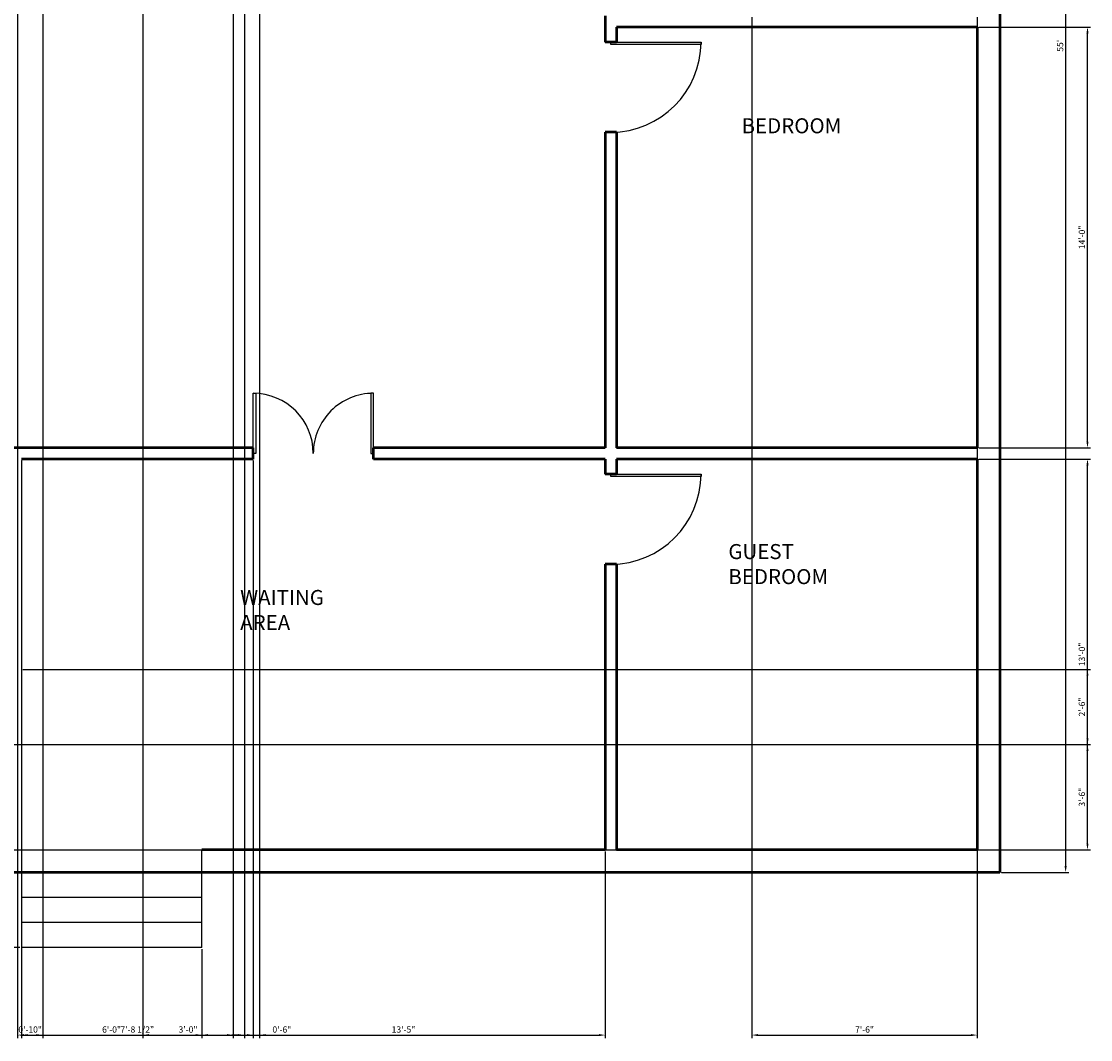
# Model space of a CAD drawing. Units: inches. Extents: x 877 to 2164, y 771 to 1603.
# Tile 3 of 6: x 1281 to 1708, y 771 to 1177. Entities that reach past the tile are written whole.
import ezdxf

# ---------------------------------------------------------------- set-up
doc = ezdxf.new("R2010")
doc.units = ezdxf.units.IN
for name, color, linetype, lineweight in [('A-ANNO-DIMS', 2, 'Continuous', 18), ('A-AREA-IDEN', 7, 'Continuous', 25), ('A-DOOR', 5, 'Continuous', 25), ('A-FLOR-STRS', 7, 'Continuous', 25), ('A-WALL', 7, 'Continuous', 50)]:
    doc.layers.add(name, color=color, linetype=linetype, lineweight=lineweight)
doc.styles.get("Standard").update_dxf_attribs({"font": 'arial.ttf'})
doc.dimstyles.new('ISO-25', dxfattribs={"dimtxt": 2.5, "dimasz": 2.5, "dimexe": 1.25, "dimexo": 0.625, "dimtad": 1, "dimdec": 0, "dimlunit": 4, "dimtxsty": 'Standard', "dimcen": 2.5, "dimadec": 0, "dimazin": 0, "dimtfac": 1, "dimtdec": 0, "dimtmove": 0, "dimatfit": 3, "dimfxl": 1, "dimarcsym": 0})

# ---------------------------------------------------------------- blocks, each defined once
blk = doc.blocks.new('*D2')
at = {"layer": 'A-ANNO-DIMS', "color": 0, "lineweight": -2, "transparency": 16777216}
for p, q in [((1672.52, 1497.62), (1699.4, 1497.62)), ((1698.15, 1495.12), (1698.15, 840.12)), ((1672.52, 837.62), (1699.4, 837.62))]:
    blk.add_line(p, q, dxfattribs=at)
at = {"layer": 'A-ANNO-DIMS', "color": 0, "transparency": 16777216}
for points in [[(1697.73, 1495.12), (1698.57, 1495.12), (1698.15, 1497.62)], [(1697.73, 840.12), (1698.57, 840.12), (1698.15, 837.62)]]:
    blk.add_solid(points, dxfattribs=at)
at = {"layer": 'Defpoints', "color": 0, "transparency": 16777216}
for p in [(1671.89, 1497.62), (1671.89, 837.62), (1698.15, 837.62)]:
    blk.add_point(p, dxfattribs=at)
at = {"layer": 'A-ANNO-DIMS', "color": 0, "transparency": 16777216, "insert": (1696.26, 1167.62), "char_height": 2.5, "attachment_point": 5, "rotation": 90}
blk.add_mtext("55'", dxfattribs=at)
blk = doc.blocks.new('DOOR-SINGLE-36IN')
blk.add_lwpolyline([(0, 0), (0, 1), (36, 1), (36, 0)], close=True)
blk.add_arc((36, 0), 36, 90, 180)
blk = doc.blocks.new('DOOR-DOUBLE-48IN')
for points in [[(0, 0), (1, 0), (1, 24), (0, 24)], [(48, 0), (47, 0), (47, 24), (48, 24)]]:
    blk.add_lwpolyline(points, close=True)
for centre, start, end in [((0, 24), 270, 0), ((48, 24), 180, 270)]:
    blk.add_arc(centre, 24, start, end)
blk = doc.blocks.new('*D18')
at = {"layer": 'A-ANNO-DIMS', "color": 0, "lineweight": -2, "transparency": 16777216}
for p, q in [((1572.89, 1179), (1572.89, 771.4)), ((1662.89, 1179), (1662.89, 771.4)), ((1575.39, 772.65), (1660.39, 772.65))]:
    blk.add_line(p, q, dxfattribs=at)
at = {"layer": 'A-ANNO-DIMS', "color": 0, "transparency": 16777216}
for points in [[(1575.39, 773.06), (1575.39, 772.23), (1572.89, 772.65)], [(1660.39, 773.06), (1660.39, 772.23), (1662.89, 772.65)]]:
    blk.add_solid(points, dxfattribs=at)
at = {"layer": 'Defpoints', "color": 0, "transparency": 16777216}
for p in [(1572.89, 1179.62), (1662.89, 1179.62), (1662.89, 772.65)]:
    blk.add_point(p, dxfattribs=at)
at = {"layer": 'A-ANNO-DIMS', "color": 0, "transparency": 16777216, "insert": (1617.89, 774.55), "char_height": 2.5, "attachment_point": 5}
blk.add_mtext('7\'-6"', dxfattribs=at)
blk = doc.blocks.new('*D22')
at = {"layer": 'A-ANNO-DIMS', "color": 0, "lineweight": -2, "transparency": 16777216}
for p, q in [((1663.52, 1175.12), (1708.12, 1175.12)), ((1706.87, 1009.62), (1706.87, 1172.62)), ((1663.52, 1007.12), (1708.12, 1007.12))]:
    blk.add_line(p, q, dxfattribs=at)
at = {"layer": 'A-ANNO-DIMS', "color": 0, "transparency": 16777216}
for points in [[(1706.45, 1172.62), (1707.29, 1172.62), (1706.87, 1175.12)], [(1706.45, 1009.62), (1707.29, 1009.62), (1706.87, 1007.12)]]:
    blk.add_solid(points, dxfattribs=at)
at = {"layer": 'Defpoints', "color": 0, "transparency": 16777216}
for p in [(1662.89, 1175.12), (1706.87, 1175.12), (1662.89, 1007.12)]:
    blk.add_point(p, dxfattribs=at)
at = {"layer": 'A-ANNO-DIMS', "color": 0, "transparency": 16777216, "insert": (1704.97, 1091.12), "char_height": 2.5, "attachment_point": 5, "rotation": 90}
blk.add_mtext('14\'-0"', dxfattribs=at)
blk = doc.blocks.new('*D23')
at = {"layer": 'A-ANNO-DIMS', "color": 0, "lineweight": -2, "transparency": 16777216}
for p, q in [((1663.52, 1002.62), (1708.12, 1002.62)), ((1706.87, 849.12), (1706.87, 1000.12)), ((1663.52, 846.62), (1708.12, 846.62))]:
    blk.add_line(p, q, dxfattribs=at)
at = {"layer": 'A-ANNO-DIMS', "color": 0, "transparency": 16777216}
for points in [[(1706.45, 1000.12), (1707.29, 1000.12), (1706.87, 1002.62)], [(1706.45, 849.12), (1707.29, 849.12), (1706.87, 846.62)]]:
    blk.add_solid(points, dxfattribs=at)
at = {"layer": 'Defpoints', "color": 0, "transparency": 16777216}
for p in [(1662.89, 1002.62), (1706.87, 1002.62), (1662.89, 846.62)]:
    blk.add_point(p, dxfattribs=at)
at = {"layer": 'A-ANNO-DIMS', "color": 0, "transparency": 16777216, "insert": (1704.97, 924.62), "char_height": 2.5, "attachment_point": 5, "rotation": 90}
blk.add_mtext('13\'-0"', dxfattribs=at)
blk = doc.blocks.new('*D27')
at = {"layer": 'A-ANNO-DIMS', "color": 0, "lineweight": -2, "transparency": 16777216}
for p, q in [((1514.39, 846), (1514.39, 771.4)), ((1353.39, 807), (1353.39, 771.4)), ((1355.89, 772.65), (1511.89, 772.65))]:
    blk.add_line(p, q, dxfattribs=at)
at = {"layer": 'A-ANNO-DIMS', "color": 0, "transparency": 16777216}
for points in [[(1355.89, 773.06), (1355.89, 772.23), (1353.39, 772.65)], [(1511.89, 773.06), (1511.89, 772.23), (1514.39, 772.65)]]:
    blk.add_solid(points, dxfattribs=at)
at = {"layer": 'Defpoints', "color": 0, "transparency": 16777216}
for p in [(1514.39, 846.62), (1353.39, 807.62), (1514.39, 772.65)]:
    blk.add_point(p, dxfattribs=at)
at = {"layer": 'A-ANNO-DIMS', "color": 0, "transparency": 16777216, "insert": (1433.89, 774.55), "char_height": 2.5, "attachment_point": 5}
blk.add_mtext('13\'-5"', dxfattribs=at)
blk = doc.blocks.new('*D29')
at = {"layer": 'A-ANNO-DIMS', "color": 0, "lineweight": -2, "transparency": 16777216}
for p, q in [((1277.52, 888.62), (1708.12, 888.62)), ((1706.87, 849.12), (1706.87, 886.12)), ((1277.52, 846.62), (1708.12, 846.62))]:
    blk.add_line(p, q, dxfattribs=at)
at = {"layer": 'A-ANNO-DIMS', "color": 0, "transparency": 16777216}
for points in [[(1706.45, 886.12), (1707.29, 886.12), (1706.87, 888.62)], [(1706.45, 849.12), (1707.29, 849.12), (1706.87, 846.62)]]:
    blk.add_solid(points, dxfattribs=at)
at = {"layer": 'Defpoints', "color": 0, "transparency": 16777216}
for p in [(1276.89, 888.62), (1706.87, 888.62), (1276.89, 846.62)]:
    blk.add_point(p, dxfattribs=at)
at = {"layer": 'A-ANNO-DIMS', "color": 0, "transparency": 16777216, "insert": (1704.97, 867.62), "char_height": 2.5, "attachment_point": 5, "rotation": 90}
blk.add_mtext('3\'-6"', dxfattribs=at)
blk = doc.blocks.new('*D30')
at = {"layer": 'A-ANNO-DIMS', "color": 0, "lineweight": -2, "transparency": 16777216}
for p, q in [((1281.39, 807), (1281.39, 771.4)), ((1353.39, 807), (1353.39, 771.4)), ((1283.89, 772.65), (1350.89, 772.65))]:
    blk.add_line(p, q, dxfattribs=at)
at = {"layer": 'A-ANNO-DIMS', "color": 0, "transparency": 16777216}
for points in [[(1283.89, 773.06), (1283.89, 772.23), (1281.39, 772.65)], [(1350.89, 773.06), (1350.89, 772.23), (1353.39, 772.65)]]:
    blk.add_solid(points, dxfattribs=at)
at = {"layer": 'Defpoints', "color": 0, "transparency": 16777216}
for p in [(1281.39, 807.62), (1353.39, 807.62), (1353.39, 772.65)]:
    blk.add_point(p, dxfattribs=at)
at = {"layer": 'A-ANNO-DIMS', "color": 0, "transparency": 16777216, "insert": (1317.39, 774.55), "char_height": 2.5, "attachment_point": 5}
blk.add_mtext('6\'-0"', dxfattribs=at)
blk = doc.blocks.new('*D31')
at = {"layer": 'A-ANNO-DIMS', "color": 0, "lineweight": -2, "transparency": 16777216}
for p, q in [((1071.27, 837.62), (1035.67, 837.62)), ((1036.92, 810.12), (1036.92, 835.12)), ((1280.77, 807.62), (1035.67, 807.62))]:
    blk.add_line(p, q, dxfattribs=at)
at = {"layer": 'A-ANNO-DIMS', "color": 0, "transparency": 16777216}
for points in [[(1036.5, 835.12), (1037.34, 835.12), (1036.92, 837.62)], [(1036.5, 810.12), (1037.34, 810.12), (1036.92, 807.62)]]:
    blk.add_solid(points, dxfattribs=at)
at = {"layer": 'Defpoints', "color": 0, "transparency": 16777216}
for p in [(1036.92, 837.62), (1071.89, 837.62), (1281.39, 807.62)]:
    blk.add_point(p, dxfattribs=at)
at = {"layer": 'A-ANNO-DIMS', "color": 0, "transparency": 16777216, "insert": (1035.02, 822.62), "char_height": 2.5, "attachment_point": 5, "rotation": 90}
blk.add_mtext('2\'-6"', dxfattribs=at)
blk = doc.blocks.new('*D36')
at = {"layer": 'A-ANNO-DIMS', "color": 0, "lineweight": -2, "transparency": 16777216}
for p, q in [((1282.02, 918.62), (1708.12, 918.62)), ((1706.87, 891.12), (1706.87, 916.12)), ((1282.02, 888.62), (1708.12, 888.62))]:
    blk.add_line(p, q, dxfattribs=at)
at = {"layer": 'A-ANNO-DIMS', "color": 0, "transparency": 16777216}
for points in [[(1706.45, 916.12), (1707.29, 916.12), (1706.87, 918.62)], [(1706.45, 891.12), (1707.29, 891.12), (1706.87, 888.62)]]:
    blk.add_solid(points, dxfattribs=at)
at = {"layer": 'Defpoints', "color": 0, "transparency": 16777216}
for p in [(1281.39, 918.62), (1706.87, 918.62), (1281.39, 888.62)]:
    blk.add_point(p, dxfattribs=at)
at = {"layer": 'A-ANNO-DIMS', "color": 0, "transparency": 16777216, "insert": (1704.97, 903.62), "char_height": 2.5, "attachment_point": 5, "rotation": 90}
blk.add_mtext('2\'-6"', dxfattribs=at)
blk = doc.blocks.new('*D42')
at = {"layer": 'A-ANNO-DIMS', "color": 0, "lineweight": -2, "transparency": 16777216}
for p, q in [((1329.89, 1362), (1329.89, 771.4)), ((1365.89, 1362), (1365.89, 771.4)), ((1332.39, 772.65), (1363.39, 772.65))]:
    blk.add_line(p, q, dxfattribs=at)
at = {"layer": 'A-ANNO-DIMS', "color": 0, "transparency": 16777216}
for points in [[(1332.39, 773.06), (1332.39, 772.23), (1329.89, 772.65)], [(1363.39, 773.06), (1363.39, 772.23), (1365.89, 772.65)]]:
    blk.add_solid(points, dxfattribs=at)
at = {"layer": 'Defpoints', "color": 0, "transparency": 16777216}
for p in [(1329.89, 1362.62), (1365.89, 1362.62), (1365.89, 772.65)]:
    blk.add_point(p, dxfattribs=at)
at = {"layer": 'A-ANNO-DIMS', "color": 0, "transparency": 16777216, "insert": (1347.89, 774.55), "char_height": 2.5, "attachment_point": 5}
blk.add_mtext('3\'-0"', dxfattribs=at)
blk = doc.blocks.new('*D44')
at = {"layer": 'A-ANNO-DIMS', "color": 0, "lineweight": -2, "transparency": 16777216}
for p, q in [((1279.89, 1452), (1279.89, 771.4)), ((1289.89, 1452), (1289.89, 771.4)), ((1282.39, 772.65), (1287.39, 772.65))]:
    blk.add_line(p, q, dxfattribs=at)
at = {"layer": 'A-ANNO-DIMS', "color": 0, "transparency": 16777216}
for points in [[(1282.39, 773.06), (1282.39, 772.23), (1279.89, 772.65)], [(1287.39, 773.06), (1287.39, 772.23), (1289.89, 772.65)]]:
    blk.add_solid(points, dxfattribs=at)
at = {"layer": 'Defpoints', "color": 0, "transparency": 16777216}
for p in [(1279.89, 1452.62), (1289.89, 1452.62), (1289.89, 772.65)]:
    blk.add_point(p, dxfattribs=at)
at = {"layer": 'A-ANNO-DIMS', "color": 0, "transparency": 16777216, "insert": (1284.89, 774.55), "char_height": 2.5, "attachment_point": 5}
blk.add_mtext('0\'-10"', dxfattribs=at)
blk = doc.blocks.new('*D45')
at = {"layer": 'A-ANNO-DIMS', "color": 0, "lineweight": -2, "transparency": 16777216}
for p, q in [((1281.39, 1002), (1281.39, 771.4)), ((1373.89, 1002), (1373.89, 771.4)), ((1283.89, 772.65), (1371.39, 772.65))]:
    blk.add_line(p, q, dxfattribs=at)
at = {"layer": 'A-ANNO-DIMS', "color": 0, "transparency": 16777216}
for points in [[(1283.89, 773.06), (1283.89, 772.23), (1281.39, 772.65)], [(1371.39, 773.06), (1371.39, 772.23), (1373.89, 772.65)]]:
    blk.add_solid(points, dxfattribs=at)
at = {"layer": 'Defpoints', "color": 0, "transparency": 16777216}
for p in [(1281.39, 1002.62), (1373.89, 1002.62), (1373.89, 772.65)]:
    blk.add_point(p, dxfattribs=at)
at = {"layer": 'A-ANNO-DIMS', "color": 0, "transparency": 16777216, "insert": (1327.64, 774.56), "char_height": 2.5, "attachment_point": 5}
blk.add_mtext('7\'-8 1/2"', dxfattribs=at)
blk = doc.blocks.new('*D46')
at = {"layer": 'A-ANNO-DIMS', "color": 0, "lineweight": -2, "transparency": 16777216}
for p, q in [((1370.39, 1344), (1370.39, 771.4)), ((1376.39, 1344), (1376.39, 771.4)), ((1367.89, 772.65), (1365.39, 772.65)), ((1370.39, 772.65), (1376.39, 772.65)), ((1378.89, 772.65), (1389.29, 772.65))]:
    blk.add_line(p, q, dxfattribs=at)
at = {"layer": 'A-ANNO-DIMS', "color": 0, "transparency": 16777216}
for points in [[(1367.89, 773.06), (1367.89, 772.23), (1370.39, 772.65)], [(1378.89, 773.06), (1378.89, 772.23), (1376.39, 772.65)]]:
    blk.add_solid(points, dxfattribs=at)
at = {"layer": 'Defpoints', "color": 0, "transparency": 16777216}
for p in [(1370.39, 1344.62), (1376.39, 1344.62), (1376.39, 772.65)]:
    blk.add_point(p, dxfattribs=at)
at = {"layer": 'A-ANNO-DIMS', "color": 0, "transparency": 16777216, "insert": (1385.34, 774.55), "char_height": 2.5, "attachment_point": 5}
blk.add_mtext('0\'-6"', dxfattribs=at)

msp = doc.modelspace()

# ---------------------------------------------------------------- linework, layer by layer
at = {"layer": 'A-FLOR-STRS'}
for p, q in [((1353.39, 807.62), (1353.39, 846.62)), ((1353.39, 827.62), (1281.39, 827.62)), ((1353.39, 817.62), (1281.39, 817.62)), ((1353.39, 807.62), (1281.39, 807.62))]:
    msp.add_line(p, q, dxfattribs=at)
at = {"layer": 'A-WALL'}
for p, q in [((1671.89, 1497.62), (1671.89, 837.62)), ((1514.39, 1179.62), (1514.39, 1169.12)), ((1518.89, 1175.12), (1518.89, 1169.12)), ((1662.89, 1175.12), (1518.89, 1175.12)), ((1662.89, 1175.12), (1662.89, 1007.12)), ((1518.89, 1169.12), (1514.39, 1169.12)), ((1518.89, 1133.12), (1514.39, 1133.12)), ((1514.39, 1133.12), (1514.39, 1007.12)), ((1518.89, 1133.12), (1518.89, 1007.12)), ((1373.89, 1007.12), (1276.89, 1007.12)), ((1373.89, 1002.62), (1373.89, 1007.12)), ((1514.39, 1007.12), (1421.89, 1007.12)), ((1421.89, 1002.62), (1421.89, 1007.12)), ((1662.89, 1007.12), (1518.89, 1007.12)), ((1373.89, 1002.62), (1281.39, 1002.62)), ((1514.39, 1002.62), (1421.89, 1002.62)), ((1514.39, 1002.62), (1514.39, 996.62)), ((1662.89, 1002.62), (1518.89, 1002.62)), ((1518.89, 1002.62), (1518.89, 996.62)), ((1662.89, 1002.62), (1662.89, 846.62)), ((1518.89, 996.62), (1514.39, 996.62)), ((1518.89, 960.62), (1514.39, 960.62)), ((1514.39, 960.62), (1514.39, 846.62)), ((1518.89, 960.62), (1518.89, 846.62)), ((1514.39, 846.62), (1353.39, 846.62)), ((1662.89, 846.62), (1518.89, 846.62)), ((1671.89, 837.62), (1071.89, 837.62))]:
    msp.add_line(p, q, dxfattribs=at)

# ---------------------------------------------------------------- block references
at = {"layer": 'A-DOOR', "rotation": 180}
for name, p in [('DOOR-SINGLE-36IN', (1552.64, 1169.12)), ('DOOR-DOUBLE-48IN', (1421.9, 1028.87)), ('DOOR-SINGLE-36IN', (1552.64, 996.62))]:
    msp.add_blockref(name, p, dxfattribs=at)

# ---------------------------------------------------------------- texts
at = {"layer": 'A-AREA-IDEN', "char_height": 6, "attachment_point": 1}
for s, insert in [('BEDROOM', (1568.82, 1138.68)), ('GUEST BEDROOM', (1563.53, 968.69)), ('WAITING AREA', (1368.7, 950.36))]:
    msp.add_mtext_dynamic_manual_height_columns(s, width=54.8109, gutter_width=12.5, heights=[0], dxfattribs=dict(at, insert=insert))

# ---------------------------------------------------------------- dimensions: what is measured, and where the dimension line sits
at = {"layer": 'A-ANNO-DIMS'}
for base, p1, p2, override, picture, middle in [((1698.15, 837.62), (1671.89, 1497.62), (1671.89, 837.62), {"dimclrd": 0, "dimclre": 0, "dimclrt": 0}, '*D2', (1696.26, 1167.62)), ((1706.87, 1175.12), (1662.89, 1007.12), (1662.89, 1175.12), {"dimdec": 1, "dimlfac": 1, "dimrnd": 0, "dimzin": 1, "dimdsep": 46, "dimlunit": 4, "dimfrac": 2}, '*D22', (1704.97, 1091.12)), ((1706.87, 1002.62), (1662.89, 846.62), (1662.89, 1002.62), {"dimdec": 1, "dimlfac": 1, "dimrnd": 0, "dimzin": 1, "dimdsep": 46, "dimlunit": 4, "dimfrac": 2}, '*D23', (1704.97, 924.62)), ((1706.87, 918.62), (1281.39, 888.62), (1281.39, 918.62), {"dimdec": 1, "dimlfac": 1, "dimrnd": 0, "dimzin": 1, "dimdsep": 46, "dimlunit": 4, "dimfrac": 2}, '*D36', (1704.97, 903.62)), ((1706.87, 888.62), (1276.89, 846.62), (1276.89, 888.62), {"dimdec": 1, "dimlfac": 1, "dimrnd": 0, "dimzin": 1, "dimdsep": 46, "dimlunit": 4, "dimfrac": 2}, '*D29', (1704.97, 867.62)), ((1036.92, 837.62), (1281.39, 807.62), (1071.89, 837.62), {"dimdec": 1, "dimlfac": 1, "dimrnd": 0, "dimzin": 1, "dimdsep": 46, "dimlunit": 4, "dimfrac": 2}, '*D31', (1035.02, 822.62))]:
    dim = msp.add_linear_dim(base=base, p1=p1, p2=p2, angle=90, dimstyle='ISO-25', override=override, dxfattribs=at)
    dim.commit()
    dim.dimension.update_dxf_attribs({"geometry": picture, "text_midpoint": middle})
for base, p1, p2, picture, middle in [((1289.89, 772.65), (1279.89, 1452.62), (1289.89, 1452.62), '*D44', (1284.89, 774.55)), ((1365.89, 772.65), (1329.89, 1362.62), (1365.89, 1362.62), '*D42', (1347.89, 774.55)), ((1376.39, 772.65), (1370.39, 1344.62), (1376.39, 1344.62), '*D46', (1385.34, 774.55)), ((1662.89, 772.65), (1572.89, 1179.62), (1662.89, 1179.62), '*D18', (1617.89, 774.55)), ((1373.89, 772.65), (1281.39, 1002.62), (1373.89, 1002.62), '*D45', (1327.64, 774.56)), ((1514.39, 772.65), (1353.39, 807.62), (1514.39, 846.62), '*D27', (1433.89, 774.55)), ((1353.39, 772.65), (1281.39, 807.62), (1353.39, 807.62), '*D30', (1317.39, 774.55))]:
    dim = msp.add_linear_dim(base=base, p1=p1, p2=p2, dimstyle='ISO-25', override={"dimdec": 1, "dimlfac": 1, "dimrnd": 0, "dimzin": 1, "dimdsep": 46, "dimlunit": 4, "dimfrac": 2}, dxfattribs=at)
    dim.commit()
    dim.dimension.update_dxf_attribs({"geometry": picture, "text_midpoint": middle})

doc.saveas('drawing.dxf')
